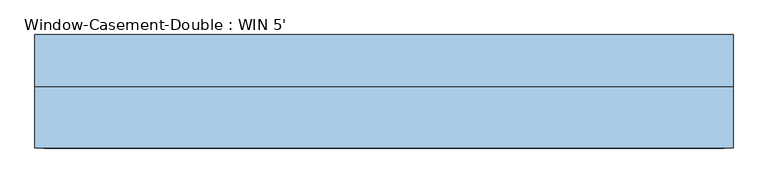
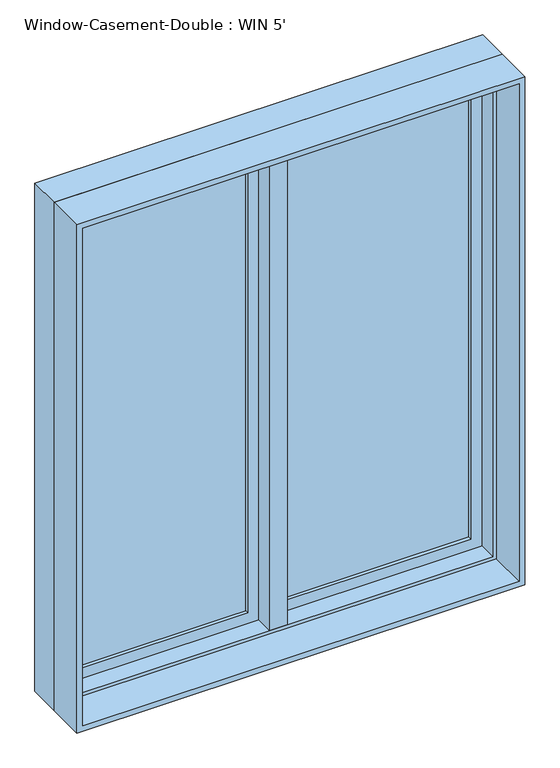
"""IFC4 building model written with IfcOpenShell, lengths in millimetres: window geometry, Window-Casement-Double : WIN 5'."""

from ifc_helpers import new_model, si_unit, frame, origin, place, context, project, spatial, polyline, outline, extrude, faceted_brep, source, transform, mapped, element, save


def window_casement_double_win_5_f93960c7(model_context):
    return source(origin(), model_context, "Body", "SolidModel", [
        faceted_brep([(9.525, 133.35, 2730.5), (-9.525, 133.35, 2730.5), (-9.525, 82.55, 2730.5), (9.525, 82.55, 2730.5), (9.525, 133.35, 927.1), (9.525, 82.55, 927.1), (-9.525, 82.55, 927.1), (-9.525, 133.35, 927.1), (-9.525, 82.55, 946.15), (-9.525, 82.55, 2711.45), (-30.1625, 82.55, 946.15), (-30.1625, 82.55, 2711.45), (-30.1625, 19.05, 946.15), (-30.1625, 19.05, 2711.45), (30.1625, 19.05, 946.15), (30.1625, 19.05, 2711.45), (30.1625, 82.55, 946.15), (30.1625, 82.55, 2711.45), (9.525, 82.55, 946.15), (9.525, 82.55, 2711.45)], [[[0, 1, 2, 3]], [[4, 5, 6, 7]], [[1, 0, 4, 7]], [[2, 1, 7, 6, 8, 9]], [[9, 8, 10, 11]], [[11, 10, 12, 13]], [[13, 12, 14, 15]], [[15, 14, 16, 17]], [[17, 16, 18, 19]], [[0, 3, 19, 18, 5, 4]], [[18, 8, 6, 5]], [[9, 19, 3, 2]], [[8, 18, 16, 14, 12, 10]], [[19, 9, 11, 13, 15, 17]]]),
        extrude(outline(polyline([(-66.675, 114.3), (-66.675, 107.95), (-692.15, 107.95), (-692.15, 114.3), (-66.675, 114.3)])), frame((0.0, 0.0, 984.25), z_axis=(0.0, 0.0, 1.0), x_axis=(1.0, 0.0, 0.0)), (0.0, 0.0, 1.0), 1689.1),
        extrude(outline(polyline([(-692.15, 95.25), (-692.15, 101.6), (-66.675, 101.6), (-66.675, 95.25), (-692.15, 95.25)])), frame((0.0, 0.0, 984.25), z_axis=(0.0, 0.0, 1.0), x_axis=(1.0, 0.0, 0.0)), (0.0, 0.0, 1.0), 1689.1),
        extrude(outline(polyline([(692.15, 114.3), (692.15, 107.95), (66.675, 107.95), (66.675, 114.3), (692.15, 114.3)])), frame((0.0, 0.0, 984.25), z_axis=(0.0, 0.0, 1.0), x_axis=(1.0, 0.0, 0.0)), (0.0, 0.0, 1.0), 1689.1),
        extrude(outline(polyline([(66.675, 95.25), (66.675, 101.6), (692.15, 101.6), (692.15, 95.25), (66.675, 95.25)])), frame((0.0, 0.0, 984.25), z_axis=(0.0, 0.0, 1.0), x_axis=(1.0, 0.0, 0.0)), (0.0, 0.0, 1.0), 1689.1),
        extrude(outline(polyline([(2730.5, -749.3), (927.1, -749.3), (927.1, -9.525), (2730.5, -9.525), (2730.5, -749.3)]), holes=[polyline([(2673.35, -66.675), (984.25, -66.675), (984.25, -692.15), (2673.35, -692.15), (2673.35, -66.675)])]), frame((0.0, 82.55, 0.0), z_axis=(0.0, 1.0, 0.0), x_axis=(0.0, 0.0, 1.0)), (0.0, 0.0, 1.0), 44.45),
        extrude(outline(polyline([(927.1, 749.3), (2730.5, 749.3), (2730.5, 9.525), (927.1, 9.525), (927.1, 749.3)]), holes=[polyline([(984.25, 66.675), (2673.35, 66.675), (2673.35, 692.15), (984.25, 692.15), (984.25, 66.675)])]), frame((0.0, 82.55, 0.0), z_axis=(0.0, 1.0, 0.0), x_axis=(0.0, 0.0, 1.0)), (0.0, 0.0, 1.0), 44.45),
        extrude(outline(polyline([(2743.2, -762.0), (914.4, -762.0), (914.4, 762.0), (2743.2, 762.0), (2743.2, -762.0)]), holes=[polyline([(2724.15, 742.95), (933.45, 742.95), (933.45, -742.95), (2724.15, -742.95), (2724.15, 742.95)])]), frame((0.0, -114.3, 0.0), z_axis=(0.0, 1.0, 0.0), x_axis=(0.0, 0.0, 1.0)), (0.0, 0.0, 1.0), 133.35),
        faceted_brep([(730.25, 82.55, 2711.45), (730.25, 19.05, 2711.45), (-730.25, 19.05, 2711.45), (-730.25, 82.55, 2711.45), (749.3, 133.35, 2730.5), (749.3, 82.55, 2730.5), (-749.3, 82.55, 2730.5), (-749.3, 133.35, 2730.5), (762.0, 19.05, 2743.2), (762.0, 133.35, 2743.2), (-762.0, 133.35, 2743.2), (-762.0, 19.05, 2743.2), (-730.25, 19.05, 946.15), (-730.25, 82.55, 946.15), (-749.3, 82.55, 927.1), (-749.3, 133.35, 927.1), (-762.0, 133.35, 914.4), (-762.0, 19.05, 914.4), (730.25, 19.05, 946.15), (730.25, 82.55, 946.15), (749.3, 82.55, 927.1), (749.3, 133.35, 927.1), (762.0, 133.35, 914.4), (762.0, 19.05, 914.4)], [[[0, 1, 2, 3]], [[4, 5, 6, 7]], [[8, 9, 10, 11]], [[3, 2, 12, 13]], [[7, 6, 14, 15]], [[11, 10, 16, 17]], [[13, 12, 18, 19]], [[15, 14, 20, 21]], [[17, 16, 22, 23]], [[11, 17, 23, 8], [1, 18, 12, 2]], [[19, 18, 1, 0]], [[5, 20, 14, 6], [3, 13, 19, 0]], [[21, 20, 5, 4]], [[23, 22, 9, 8]], [[9, 22, 16, 10], [7, 15, 21, 4]]]),
    ])


if __name__ == "__main__":
    model = new_model("IFC4")
    model_context = context("Model", 3, world=origin())
    ifc_project = project(units=[si_unit("LENGTHUNIT", "METRE", prefix="MILLI")], contexts=[model_context])
    site = spatial("IfcSite", under=ifc_project)
    building = spatial("IfcBuilding", under=site)
    placement = place(None, origin())
    window_casement_double_win_5_shape = window_casement_double_win_5_f93960c7(model_context)
    element("IfcWindow", 1, ObjectType="Window-Casement-Double : WIN 5'", at=placement, inside=building, context=model_context, shape_type="MappedRepresentation", body=[
        mapped(window_casement_double_win_5_shape, transform((0.0, 0.0, 0.0), x_axis=(1.0, 0.0, 0.0), y_axis=(0.0, 1.0, 0.0), z_axis=(0.0, 0.0, 1.0))),
    ])
    save(model, "model.ifc")

# Revit data of these elements
# Type "Window-Casement-Double : WIN 5'"
#   Type Mark = "20"
#   Fire Rating = "0.5h"
#   Assembly Code = "B2020100"
#   Analytic Construction = "Double glazing - domestic"
#   Frame Extension [instance default] = 0' - 0 1/4"
#   Window Inset [instance default] = 0' - 0"
#   Wall Thickness [instance default] = 0' - 6"
#   Interior Wall Closure [instance default] = 0' - 2 1/4"
#   Half Width = 2' - 6"
#   Visual Light Transmittance = 0.81
#   Thermal Resistance (R) = 1.8146 (h·ft²·°F)/BTU
#   Solar Heat Gain Coefficient = 0.76
#   Rough Width = 5' - 0 1/2"
#   Rough Height = 6' - 0 1/2"
#   Height = 6' - 0"
#   Heat Transfer Coefficient (U) = 0.5511 BTU/(h·ft²·°F)
#   Exterior Wall Closure [instance default] = 0' - 1 1/4"
#   Extension Jamb [instance default] = 0' - 2 1/4"
#   Default Sill Height = 3' - 0"
#   Width = 5' - 0"
#   Muntin Visibility = yes
#   Interior Trim Visibility [instance default] = yes
#   Exterior Trim Visibility [instance default] = yes
#   Extension Jamb Visibility [instance default] = yes
#   Interior Trim Material = Wood - Stained
#   Muntin Pattern = Muntin Pattern_2x2 : Muntin Pattern_2x2
#   Interior Trim = Trim-Window-Interior-Flat : Picture Frame
#   Interior Frame Material = Wood - Stained
#   Glass Panel Material = Glass
#   Exterior Trim Material = Clad - White
#   Exterior Trim = Trim-Window-Exterior-Flat : with Sill
#   Exterior Frame Material = Clad - White
#   Wall Closure = (empty or 0)
# Element 1 (IfcWindow, "Window-Casement-Double : WIN 5'")
#   Wall Thickness = 0' - 9"
#   Extension Jamb = 0' - 5 1/4"
#   Materials on its faces: "Wood - Stained", "Glass", "Clad - White"
# Materials
#   "Wood - Stained": class "Wood", colour RGB 224 178 126, transparency 0, Cost = 0
#   "Glass": class "Glass", colour RGB 0 128 192, transparency 0.75, Description = "Soda Lime Glass", Cost = 0
#   "Clad - White": class "Wood", colour RGB 242 242 238, transparency 0, Cost = 0
